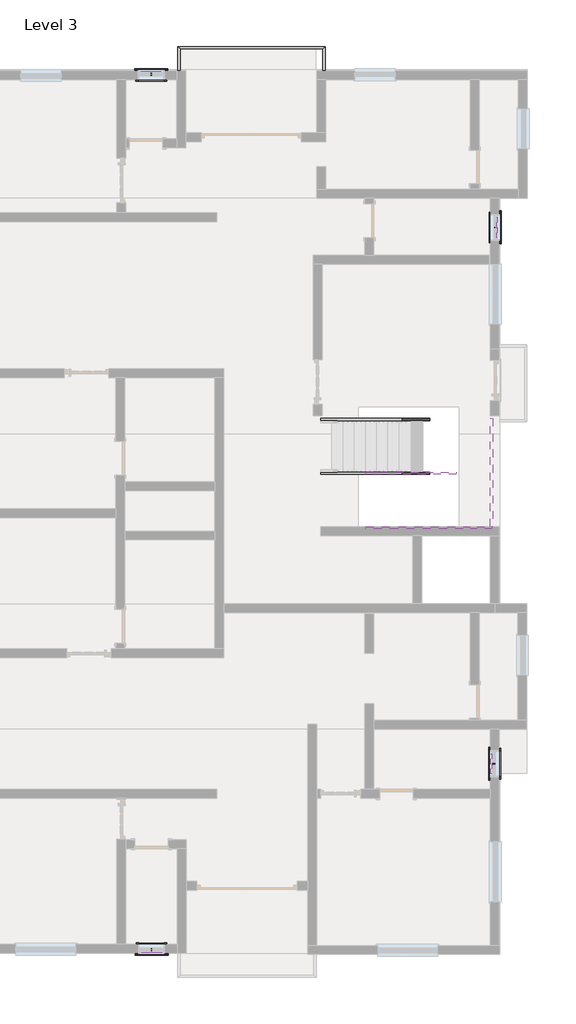
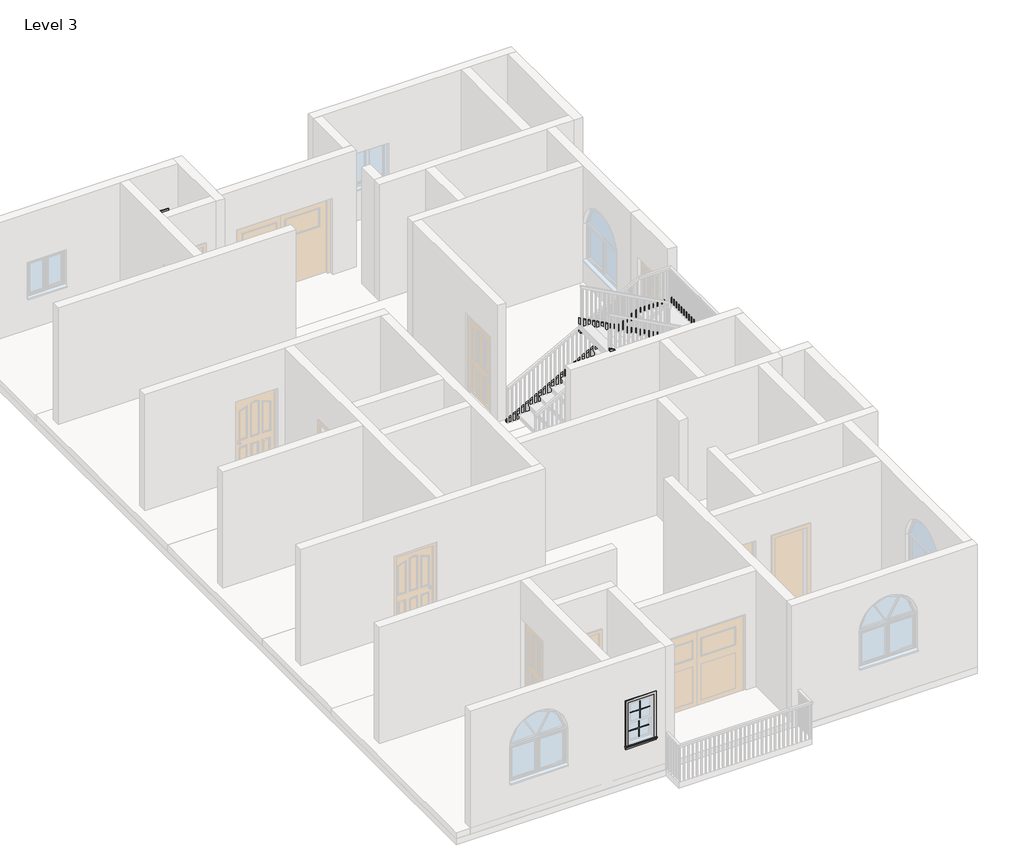
# One storey, part 7 of 7: 16 proxies, 5 members, 1 railing.
"""IFC4 building model written with IfcOpenShell, lengths in millimetres."""

from ifc_helpers import new_model, si_unit, frame, origin, place, context, project, spatial, polyline, outline, extrude, faceted_brep, transform, mapped, element, save
from components import muntin_pattern_2x2_muntin_pattern_2x2_eba6c5fb, trim_window_exterior_flat_with_sill_278e6a94, trim_window_interior_flat_picture_frame_e9fd5f45

model = new_model("IFC4")

# Units and contexts
model_context = context("Model", 3, world=origin())
ifc_project = project(units=[si_unit("LENGTHUNIT", "METRE", prefix="MILLI")], contexts=[model_context])

# Site, building, storey
site = spatial("IfcSite", under=ifc_project)
building = spatial("IfcBuilding", under=site)
storey = spatial("IfcBuildingStorey", under=building, Name="Level 3", Elevation=6096.0)

# Proxies
placement = place(None, origin())
muntin_pattern_2x2_muntin_pattern_2x2_shape = muntin_pattern_2x2_muntin_pattern_2x2_eba6c5fb(model_context)
element("IfcBuildingElementProxy", 1, Name="Muntin Pattern_2x2 : Muntin Pattern_2x2", ObjectType="Muntin Pattern_2x2 : Muntin Pattern_2x2", at=placement, inside=storey, context=model_context, shape_type="MappedRepresentation", body=[
    mapped(muntin_pattern_2x2_muntin_pattern_2x2_shape, transform((5828.2640963, 5846.2962251, 7566.025), x_axis=(0.0, -1.0, 0.0), y_axis=(1.0, 0.0, 0.0), z_axis=(0.0, 0.0, 1.0))),
])
element("IfcBuildingElementProxy", 2, Name="Muntin Pattern_2x2 : Muntin Pattern_2x2", ObjectType="Muntin Pattern_2x2 : Muntin Pattern_2x2", at=placement, inside=storey, context=model_context, shape_type="MappedRepresentation", body=[
    mapped(muntin_pattern_2x2_muntin_pattern_2x2_shape, transform((5783.8140963, 5846.2962251, 7086.6), x_axis=(0.0, -1.0, 0.0), y_axis=(1.0, 0.0, 0.0), z_axis=(0.0, 0.0, 1.0))),
])
element("IfcBuildingElementProxy", 3, Name="Muntin Pattern_2x2 : Muntin Pattern_2x2", ObjectType="Muntin Pattern_2x2 : Muntin Pattern_2x2", at=placement, inside=storey, context=model_context, shape_type="MappedRepresentation", body=[
    mapped(muntin_pattern_2x2_muntin_pattern_2x2_shape, transform((5694.9140963, -6313.9537749, 7566.025), x_axis=(0.0, 1.0, 0.0), y_axis=(-1.0, 0.0, 0.0), z_axis=(0.0, 0.0, 1.0))),
])
element("IfcBuildingElementProxy", 4, Name="Muntin Pattern_2x2 : Muntin Pattern_2x2", ObjectType="Muntin Pattern_2x2 : Muntin Pattern_2x2", at=placement, inside=storey, context=model_context, shape_type="MappedRepresentation", body=[
    mapped(muntin_pattern_2x2_muntin_pattern_2x2_shape, transform((5739.3640963, -6313.9537749, 7086.6), x_axis=(0.0, 1.0, 0.0), y_axis=(-1.0, 0.0, 0.0), z_axis=(0.0, 0.0, 1.0))),
])
element("IfcBuildingElementProxy", 5, Name="Muntin Pattern_2x2 : Muntin Pattern_2x2", ObjectType="Muntin Pattern_2x2 : Muntin Pattern_2x2", at=placement, inside=storey, context=model_context, shape_type="MappedRepresentation", body=[
    mapped(muntin_pattern_2x2_muntin_pattern_2x2_shape, transform((-2029.8609037, 9366.9277313, 7566.025), x_axis=(1.0, 0.0, 0.0), y_axis=(0.0, 1.0, 0.0), z_axis=(0.0, 0.0, 1.0))),
])
element("IfcBuildingElementProxy", 6, Name="Muntin Pattern_2x2 : Muntin Pattern_2x2", ObjectType="Muntin Pattern_2x2 : Muntin Pattern_2x2", at=placement, inside=storey, context=model_context, shape_type="MappedRepresentation", body=[
    mapped(muntin_pattern_2x2_muntin_pattern_2x2_shape, transform((-2029.8609037, 9322.4777313, 7086.6), x_axis=(1.0, 0.0, 0.0), y_axis=(0.0, 1.0, 0.0), z_axis=(0.0, 0.0, 1.0))),
])
element("IfcBuildingElementProxy", 7, Name="Muntin Pattern_2x2 : Muntin Pattern_2x2", ObjectType="Muntin Pattern_2x2 : Muntin Pattern_2x2", at=placement, inside=storey, context=model_context, shape_type="MappedRepresentation", body=[
    mapped(muntin_pattern_2x2_muntin_pattern_2x2_shape, transform((-2023.5109037, -10577.9787749, 7566.025), x_axis=(-1.0, 0.0, 0.0), y_axis=(0.0, -1.0, 0.0), z_axis=(0.0, 0.0, 1.0))),
])
element("IfcBuildingElementProxy", 8, Name="Muntin Pattern_2x2 : Muntin Pattern_2x2", ObjectType="Muntin Pattern_2x2 : Muntin Pattern_2x2", at=placement, inside=storey, context=model_context, shape_type="MappedRepresentation", body=[
    mapped(muntin_pattern_2x2_muntin_pattern_2x2_shape, transform((-2023.5109037, -10533.5287749, 7086.6), x_axis=(-1.0, 0.0, 0.0), y_axis=(0.0, -1.0, 0.0), z_axis=(0.0, 0.0, 1.0))),
])
trim_window_exterior_flat_with_sill_shape = trim_window_exterior_flat_with_sill_278e6a94(model_context)
element("IfcBuildingElementProxy", 9, Name="Trim-Window-Exterior-Flat : with Sill", ObjectType="Trim-Window-Exterior-Flat : with Sill", at=placement, inside=storey, context=model_context, shape_type="MappedRepresentation", body=[
    mapped(trim_window_exterior_flat_with_sill_shape, transform((5863.1890963, 5846.2962251, 8077.2), x_axis=(0.0, 1.0, 0.0), y_axis=(0.0, 0.0, 1.0), z_axis=(1.0, 0.0, 0.0))),
])
element("IfcBuildingElementProxy", 10, Name="Trim-Window-Exterior-Flat : with Sill", ObjectType="Trim-Window-Exterior-Flat : with Sill", at=placement, inside=storey, context=model_context, shape_type="MappedRepresentation", body=[
    mapped(trim_window_exterior_flat_with_sill_shape, transform((5659.9890963, -6313.9537749, 8077.2), x_axis=(0.0, -1.0, 0.0), y_axis=(0.0, 0.0, 1.0), z_axis=(-1.0, 0.0, 0.0))),
])
element("IfcBuildingElementProxy", 11, Name="Trim-Window-Exterior-Flat : with Sill", ObjectType="Trim-Window-Exterior-Flat : with Sill", at=placement, inside=storey, context=model_context, shape_type="MappedRepresentation", body=[
    mapped(trim_window_exterior_flat_with_sill_shape, transform((-2029.8609037, 9401.8527313, 8077.2), x_axis=(-1.0, 0.0, 0.0), y_axis=(0.0, 0.0, 1.0), z_axis=(0.0, 1.0, 0.0))),
])
element("IfcBuildingElementProxy", 12, Name="Trim-Window-Exterior-Flat : with Sill", ObjectType="Trim-Window-Exterior-Flat : with Sill", at=placement, inside=storey, context=model_context, shape_type="MappedRepresentation", body=[
    mapped(trim_window_exterior_flat_with_sill_shape, transform((-2023.5109037, -10612.9037749, 8077.2), x_axis=(1.0, 0.0, 0.0), y_axis=(0.0, 0.0, 1.0), z_axis=(0.0, -1.0, 0.0))),
])
trim_window_interior_flat_picture_frame_shape = trim_window_interior_flat_picture_frame_e9fd5f45(model_context)
element("IfcBuildingElementProxy", 13, Name="Trim-Window-Interior-Flat : Picture Frame", ObjectType="Trim-Window-Interior-Flat : Picture Frame", at=placement, inside=storey, context=model_context, shape_type="MappedRepresentation", body=[
    mapped(trim_window_interior_flat_picture_frame_shape, transform((5659.9890963, 5846.2962251, 8077.2), x_axis=(0.0, -1.0, 0.0), y_axis=(0.0, 0.0, 1.0), z_axis=(-1.0, 0.0, 0.0))),
])
element("IfcBuildingElementProxy", 14, Name="Trim-Window-Interior-Flat : Picture Frame", ObjectType="Trim-Window-Interior-Flat : Picture Frame", at=placement, inside=storey, context=model_context, shape_type="MappedRepresentation", body=[
    mapped(trim_window_interior_flat_picture_frame_shape, transform((5863.1890963, -6313.9537749, 8077.2), x_axis=(0.0, 1.0, 0.0), y_axis=(0.0, 0.0, 1.0), z_axis=(1.0, 0.0, 0.0))),
])
element("IfcBuildingElementProxy", 15, Name="Trim-Window-Interior-Flat : Picture Frame", ObjectType="Trim-Window-Interior-Flat : Picture Frame", at=placement, inside=storey, context=model_context, shape_type="MappedRepresentation", body=[
    mapped(trim_window_interior_flat_picture_frame_shape, transform((-2029.8609037, 9198.6527313, 8077.2), x_axis=(1.0, 0.0, 0.0), y_axis=(0.0, 0.0, 1.0), z_axis=(0.0, -1.0, 0.0))),
])
element("IfcBuildingElementProxy", 16, Name="Trim-Window-Interior-Flat : Picture Frame", ObjectType="Trim-Window-Interior-Flat : Picture Frame", at=placement, inside=storey, context=model_context, shape_type="MappedRepresentation", body=[
    mapped(trim_window_interior_flat_picture_frame_shape, transform((-2023.5109037, -10409.7037749, 8077.2), x_axis=(-1.0, 0.0, 0.0), y_axis=(0.0, 0.0, 1.0), z_axis=(0.0, 1.0, 0.0))),
])

# Members
element("IfcMember", 17, ObjectType="Stringer - 2\" Width", at=placement, inside=storey, context=model_context, shape_type="SweptSolid", body=[
    extrude(outline(polyline([(6303.4423129, 1811.8890963), (6096.0, 1811.8890963), (6096.0, 2068.9379367), (7973.2909091, 5536.6829612), (7973.2909091, 4896.4452154), (6303.4423129, 1811.8890963)])), frame((0.0, 1464.7962251, 0.0), z_axis=(0.0, 1.0, 0.0), x_axis=(0.0, 0.0, 1.0)), (0.0, 0.0, 1.0), 50.8),
])
element("IfcMember", 18, ObjectType="Stringer - 2\" Width", at=placement, inside=storey, context=model_context, shape_type="SweptSolid", body=[
    extrude(outline(polyline([(5659.9890963, 1515.5962251), (5710.7890963, 1515.5962251), (5710.7890963, -935.5037749), (5659.9890963, -935.5037749), (5659.9890963, 1515.5962251)])), frame((0.0, 0.0, 7668.4909091), z_axis=(0.0, 0.0, 1.0), x_axis=(1.0, 0.0, 0.0)), (0.0, 0.0, 1.0), 304.8),
])
element("IfcMember", 19, ObjectType="Stringer - 2\" Width", at=placement, inside=storey, context=model_context, shape_type="SweptSolid", body=[
    extrude(outline(polyline([(7668.4909091, 5687.6636359), (9210.0362324, 2827.8890963), (8863.7736638, 2827.8890963), (7668.4909091, 5045.2998579), (7668.4909091, 5687.6636359)])), frame((0.0, -986.3037749, 0.0), z_axis=(0.0, 1.0, 0.0), x_axis=(0.0, 0.0, 1.0)), (0.0, 0.0, 1.0), 50.8),
])
element("IfcMember", 20, ObjectType="Stringer - 2\" Width", at=placement, inside=storey, context=model_context, shape_type="SweptSolid", body=[
    extrude(outline(polyline([(6303.4423129, 1811.8890963), (6096.0, 1811.8890963), (6096.0, 2068.9379367), (7590.8485088, 4830.2326586), (7937.4462232, 4830.2326586), (6303.4423129, 1811.8890963)])), frame((0.0, 245.5962251, 0.0), z_axis=(0.0, 1.0, 0.0), x_axis=(0.0, 0.0, 1.0)), (0.0, 0.0, 1.0), 50.8),
])
element("IfcMember", 21, ObjectType="Stringer - 2\" Width", at=placement, inside=storey, context=model_context, shape_type="SweptSolid", body=[
    extrude(outline(polyline([(7757.0382157, 4881.0326586), (8103.3007843, 4881.0326586), (9210.0362324, 2827.8890963), (8863.7736638, 2827.8890963), (7757.0382157, 4881.0326586)])), frame((0.0, 245.5962251, 0.0), z_axis=(0.0, 1.0, 0.0), x_axis=(0.0, 0.0, 1.0)), (0.0, 0.0, 1.0), 50.8),
])

# Railing
element("IfcRailing", 22, ObjectType="Handrail - Rectangular", at=placement, inside=storey, context=model_context, shape_type="SolidModel", body=[
    faceted_brep([(-1426.6109037, 9402.2962251, 7010.4), (-1426.6109037, 9402.2962251, 6959.6), (-1375.8109037, 9402.2962251, 6959.6), (-1375.8109037, 9402.2962251, 7010.4), (-1426.6109037, 9948.3962251, 7010.4), (-1426.6109037, 9948.3962251, 6959.6), (-1375.8109037, 9897.5962251, 6959.6), (-1375.8109037, 9897.5962251, 7010.4), (1913.4890963, 9948.3962251, 7010.4), (1913.4890963, 9948.3962251, 6959.6), (1862.6890963, 9897.5962251, 6959.6), (1862.6890963, 9897.5962251, 7010.4), (1913.4890963, 9402.2962251, 7010.4), (1862.6890963, 9402.2962251, 7010.4), (1862.6890963, 9402.2962251, 6959.6), (1913.4890963, 9402.2962251, 6959.6)], [[[0, 1, 2, 3]], [[1, 0, 4, 5]], [[2, 1, 5, 6]], [[3, 2, 6, 7]], [[0, 3, 7, 4]], [[5, 4, 8, 9]], [[6, 5, 9, 10]], [[7, 6, 10, 11]], [[4, 7, 11, 8]], [[12, 13, 14, 15]], [[9, 8, 12, 15]], [[10, 9, 15, 14]], [[11, 10, 14, 13]], [[8, 11, 13, 12]]]),
    extrude(outline(polyline([(1878.5640963, 9424.5212251), (1897.6140963, 9424.5212251), (1897.6140963, 9405.4712251), (1878.5640963, 9405.4712251), (1878.5640963, 9424.5212251)])), frame((0.0, 0.0, 6096.0), z_axis=(0.0, 0.0, 1.0), x_axis=(1.0, 0.0, 0.0)), (0.0, 0.0, 1.0), 863.6),
    extrude(outline(polyline([(1878.5640963, 9526.1212251), (1897.6140963, 9526.1212251), (1897.6140963, 9507.0712251), (1878.5640963, 9507.0712251), (1878.5640963, 9526.1212251)])), frame((0.0, 0.0, 6096.0), z_axis=(0.0, 0.0, 1.0), x_axis=(1.0, 0.0, 0.0)), (0.0, 0.0, 1.0), 863.6),
    extrude(outline(polyline([(1878.5640963, 9627.7212251), (1897.6140963, 9627.7212251), (1897.6140963, 9608.6712251), (1878.5640963, 9608.6712251), (1878.5640963, 9627.7212251)])), frame((0.0, 0.0, 6096.0), z_axis=(0.0, 0.0, 1.0), x_axis=(1.0, 0.0, 0.0)), (0.0, 0.0, 1.0), 863.6),
    extrude(outline(polyline([(1878.5640963, 9729.3212251), (1897.6140963, 9729.3212251), (1897.6140963, 9710.2712251), (1878.5640963, 9710.2712251), (1878.5640963, 9729.3212251)])), frame((0.0, 0.0, 6096.0), z_axis=(0.0, 0.0, 1.0), x_axis=(1.0, 0.0, 0.0)), (0.0, 0.0, 1.0), 863.6),
    extrude(outline(polyline([(1878.5640963, 9830.9212251), (1897.6140963, 9830.9212251), (1897.6140963, 9811.8712251), (1878.5640963, 9811.8712251), (1878.5640963, 9830.9212251)])), frame((0.0, 0.0, 6096.0), z_axis=(0.0, 0.0, 1.0), x_axis=(1.0, 0.0, 0.0)), (0.0, 0.0, 1.0), 863.6),
    extrude(outline(polyline([(1840.4640963, 9913.4712251), (1840.4640963, 9932.5212251), (1859.5140963, 9932.5212251), (1859.5140963, 9913.4712251), (1840.4640963, 9913.4712251)])), frame((0.0, 0.0, 6096.0), z_axis=(0.0, 0.0, 1.0), x_axis=(1.0, 0.0, 0.0)), (0.0, 0.0, 1.0), 863.6),
    extrude(outline(polyline([(1738.8640963, 9913.4712251), (1738.8640963, 9932.5212251), (1757.9140963, 9932.5212251), (1757.9140963, 9913.4712251), (1738.8640963, 9913.4712251)])), frame((0.0, 0.0, 6096.0), z_axis=(0.0, 0.0, 1.0), x_axis=(1.0, 0.0, 0.0)), (0.0, 0.0, 1.0), 863.6),
    extrude(outline(polyline([(1637.2640963, 9913.4712251), (1637.2640963, 9932.5212251), (1656.3140963, 9932.5212251), (1656.3140963, 9913.4712251), (1637.2640963, 9913.4712251)])), frame((0.0, 0.0, 6096.0), z_axis=(0.0, 0.0, 1.0), x_axis=(1.0, 0.0, 0.0)), (0.0, 0.0, 1.0), 863.6),
    extrude(outline(polyline([(1535.6640963, 9913.4712251), (1535.6640963, 9932.5212251), (1554.7140963, 9932.5212251), (1554.7140963, 9913.4712251), (1535.6640963, 9913.4712251)])), frame((0.0, 0.0, 6096.0), z_axis=(0.0, 0.0, 1.0), x_axis=(1.0, 0.0, 0.0)), (0.0, 0.0, 1.0), 863.6),
    extrude(outline(polyline([(1434.0640963, 9913.4712251), (1434.0640963, 9932.5212251), (1453.1140963, 9932.5212251), (1453.1140963, 9913.4712251), (1434.0640963, 9913.4712251)])), frame((0.0, 0.0, 6096.0), z_axis=(0.0, 0.0, 1.0), x_axis=(1.0, 0.0, 0.0)), (0.0, 0.0, 1.0), 863.6),
    extrude(outline(polyline([(1332.4640963, 9913.4712251), (1332.4640963, 9932.5212251), (1351.5140963, 9932.5212251), (1351.5140963, 9913.4712251), (1332.4640963, 9913.4712251)])), frame((0.0, 0.0, 6096.0), z_axis=(0.0, 0.0, 1.0), x_axis=(1.0, 0.0, 0.0)), (0.0, 0.0, 1.0), 863.6),
    extrude(outline(polyline([(1230.8640963, 9913.4712251), (1230.8640963, 9932.5212251), (1249.9140963, 9932.5212251), (1249.9140963, 9913.4712251), (1230.8640963, 9913.4712251)])), frame((0.0, 0.0, 6096.0), z_axis=(0.0, 0.0, 1.0), x_axis=(1.0, 0.0, 0.0)), (0.0, 0.0, 1.0), 863.6),
    extrude(outline(polyline([(1129.2640963, 9913.4712251), (1129.2640963, 9932.5212251), (1148.3140963, 9932.5212251), (1148.3140963, 9913.4712251), (1129.2640963, 9913.4712251)])), frame((0.0, 0.0, 6096.0), z_axis=(0.0, 0.0, 1.0), x_axis=(1.0, 0.0, 0.0)), (0.0, 0.0, 1.0), 863.6),
    extrude(outline(polyline([(1027.6640963, 9913.4712251), (1027.6640963, 9932.5212251), (1046.7140963, 9932.5212251), (1046.7140963, 9913.4712251), (1027.6640963, 9913.4712251)])), frame((0.0, 0.0, 6096.0), z_axis=(0.0, 0.0, 1.0), x_axis=(1.0, 0.0, 0.0)), (0.0, 0.0, 1.0), 863.6),
    extrude(outline(polyline([(926.0640963, 9913.4712251), (926.0640963, 9932.5212251), (945.1140963, 9932.5212251), (945.1140963, 9913.4712251), (926.0640963, 9913.4712251)])), frame((0.0, 0.0, 6096.0), z_axis=(0.0, 0.0, 1.0), x_axis=(1.0, 0.0, 0.0)), (0.0, 0.0, 1.0), 863.6),
    extrude(outline(polyline([(824.4640963, 9913.4712251), (824.4640963, 9932.5212251), (843.5140963, 9932.5212251), (843.5140963, 9913.4712251), (824.4640963, 9913.4712251)])), frame((0.0, 0.0, 6096.0), z_axis=(0.0, 0.0, 1.0), x_axis=(1.0, 0.0, 0.0)), (0.0, 0.0, 1.0), 863.6),
    extrude(outline(polyline([(722.8640963, 9913.4712251), (722.8640963, 9932.5212251), (741.9140963, 9932.5212251), (741.9140963, 9913.4712251), (722.8640963, 9913.4712251)])), frame((0.0, 0.0, 6096.0), z_axis=(0.0, 0.0, 1.0), x_axis=(1.0, 0.0, 0.0)), (0.0, 0.0, 1.0), 863.6),
    extrude(outline(polyline([(621.2640963, 9913.4712251), (621.2640963, 9932.5212251), (640.3140963, 9932.5212251), (640.3140963, 9913.4712251), (621.2640963, 9913.4712251)])), frame((0.0, 0.0, 6096.0), z_axis=(0.0, 0.0, 1.0), x_axis=(1.0, 0.0, 0.0)), (0.0, 0.0, 1.0), 863.6),
    extrude(outline(polyline([(519.6640963, 9913.4712251), (519.6640963, 9932.5212251), (538.7140963, 9932.5212251), (538.7140963, 9913.4712251), (519.6640963, 9913.4712251)])), frame((0.0, 0.0, 6096.0), z_axis=(0.0, 0.0, 1.0), x_axis=(1.0, 0.0, 0.0)), (0.0, 0.0, 1.0), 863.6),
    extrude(outline(polyline([(418.0640963, 9913.4712251), (418.0640963, 9932.5212251), (437.1140963, 9932.5212251), (437.1140963, 9913.4712251), (418.0640963, 9913.4712251)])), frame((0.0, 0.0, 6096.0), z_axis=(0.0, 0.0, 1.0), x_axis=(1.0, 0.0, 0.0)), (0.0, 0.0, 1.0), 863.6),
    extrude(outline(polyline([(316.4640963, 9913.4712251), (316.4640963, 9932.5212251), (335.5140963, 9932.5212251), (335.5140963, 9913.4712251), (316.4640963, 9913.4712251)])), frame((0.0, 0.0, 6096.0), z_axis=(0.0, 0.0, 1.0), x_axis=(1.0, 0.0, 0.0)), (0.0, 0.0, 1.0), 863.6),
    extrude(outline(polyline([(214.8640963, 9913.4712251), (214.8640963, 9932.5212251), (233.9140963, 9932.5212251), (233.9140963, 9913.4712251), (214.8640963, 9913.4712251)])), frame((0.0, 0.0, 6096.0), z_axis=(0.0, 0.0, 1.0), x_axis=(1.0, 0.0, 0.0)), (0.0, 0.0, 1.0), 863.6),
    extrude(outline(polyline([(113.2640963, 9913.4712251), (113.2640963, 9932.5212251), (132.3140963, 9932.5212251), (132.3140963, 9913.4712251), (113.2640963, 9913.4712251)])), frame((0.0, 0.0, 6096.0), z_axis=(0.0, 0.0, 1.0), x_axis=(1.0, 0.0, 0.0)), (0.0, 0.0, 1.0), 863.6),
    extrude(outline(polyline([(11.6640963, 9913.4712251), (11.6640963, 9932.5212251), (30.7140963, 9932.5212251), (30.7140963, 9913.4712251), (11.6640963, 9913.4712251)])), frame((0.0, 0.0, 6096.0), z_axis=(0.0, 0.0, 1.0), x_axis=(1.0, 0.0, 0.0)), (0.0, 0.0, 1.0), 863.6),
    extrude(outline(polyline([(-89.9359037, 9913.4712251), (-89.9359037, 9932.5212251), (-70.8859037, 9932.5212251), (-70.8859037, 9913.4712251), (-89.9359037, 9913.4712251)])), frame((0.0, 0.0, 6096.0), z_axis=(0.0, 0.0, 1.0), x_axis=(1.0, 0.0, 0.0)), (0.0, 0.0, 1.0), 863.6),
    extrude(outline(polyline([(-191.5359037, 9913.4712251), (-191.5359037, 9932.5212251), (-172.4859037, 9932.5212251), (-172.4859037, 9913.4712251), (-191.5359037, 9913.4712251)])), frame((0.0, 0.0, 6096.0), z_axis=(0.0, 0.0, 1.0), x_axis=(1.0, 0.0, 0.0)), (0.0, 0.0, 1.0), 863.6),
    extrude(outline(polyline([(-293.1359037, 9913.4712251), (-293.1359037, 9932.5212251), (-274.0859037, 9932.5212251), (-274.0859037, 9913.4712251), (-293.1359037, 9913.4712251)])), frame((0.0, 0.0, 6096.0), z_axis=(0.0, 0.0, 1.0), x_axis=(1.0, 0.0, 0.0)), (0.0, 0.0, 1.0), 863.6),
    extrude(outline(polyline([(-394.7359037, 9913.4712251), (-394.7359037, 9932.5212251), (-375.6859037, 9932.5212251), (-375.6859037, 9913.4712251), (-394.7359037, 9913.4712251)])), frame((0.0, 0.0, 6096.0), z_axis=(0.0, 0.0, 1.0), x_axis=(1.0, 0.0, 0.0)), (0.0, 0.0, 1.0), 863.6),
    extrude(outline(polyline([(-496.3359037, 9913.4712251), (-496.3359037, 9932.5212251), (-477.2859037, 9932.5212251), (-477.2859037, 9913.4712251), (-496.3359037, 9913.4712251)])), frame((0.0, 0.0, 6096.0), z_axis=(0.0, 0.0, 1.0), x_axis=(1.0, 0.0, 0.0)), (0.0, 0.0, 1.0), 863.6),
    extrude(outline(polyline([(-597.9359037, 9913.4712251), (-597.9359037, 9932.5212251), (-578.8859037, 9932.5212251), (-578.8859037, 9913.4712251), (-597.9359037, 9913.4712251)])), frame((0.0, 0.0, 6096.0), z_axis=(0.0, 0.0, 1.0), x_axis=(1.0, 0.0, 0.0)), (0.0, 0.0, 1.0), 863.6),
    extrude(outline(polyline([(-699.5359037, 9913.4712251), (-699.5359037, 9932.5212251), (-680.4859037, 9932.5212251), (-680.4859037, 9913.4712251), (-699.5359037, 9913.4712251)])), frame((0.0, 0.0, 6096.0), z_axis=(0.0, 0.0, 1.0), x_axis=(1.0, 0.0, 0.0)), (0.0, 0.0, 1.0), 863.6),
    extrude(outline(polyline([(-801.1359037, 9913.4712251), (-801.1359037, 9932.5212251), (-782.0859037, 9932.5212251), (-782.0859037, 9913.4712251), (-801.1359037, 9913.4712251)])), frame((0.0, 0.0, 6096.0), z_axis=(0.0, 0.0, 1.0), x_axis=(1.0, 0.0, 0.0)), (0.0, 0.0, 1.0), 863.6),
    extrude(outline(polyline([(-902.7359037, 9913.4712251), (-902.7359037, 9932.5212251), (-883.6859037, 9932.5212251), (-883.6859037, 9913.4712251), (-902.7359037, 9913.4712251)])), frame((0.0, 0.0, 6096.0), z_axis=(0.0, 0.0, 1.0), x_axis=(1.0, 0.0, 0.0)), (0.0, 0.0, 1.0), 863.6),
    extrude(outline(polyline([(-1004.3359037, 9913.4712251), (-1004.3359037, 9932.5212251), (-985.2859037, 9932.5212251), (-985.2859037, 9913.4712251), (-1004.3359037, 9913.4712251)])), frame((0.0, 0.0, 6096.0), z_axis=(0.0, 0.0, 1.0), x_axis=(1.0, 0.0, 0.0)), (0.0, 0.0, 1.0), 863.6),
    extrude(outline(polyline([(-1105.9359037, 9913.4712251), (-1105.9359037, 9932.5212251), (-1086.8859037, 9932.5212251), (-1086.8859037, 9913.4712251), (-1105.9359037, 9913.4712251)])), frame((0.0, 0.0, 6096.0), z_axis=(0.0, 0.0, 1.0), x_axis=(1.0, 0.0, 0.0)), (0.0, 0.0, 1.0), 863.6),
    extrude(outline(polyline([(-1207.5359037, 9913.4712251), (-1207.5359037, 9932.5212251), (-1188.4859037, 9932.5212251), (-1188.4859037, 9913.4712251), (-1207.5359037, 9913.4712251)])), frame((0.0, 0.0, 6096.0), z_axis=(0.0, 0.0, 1.0), x_axis=(1.0, 0.0, 0.0)), (0.0, 0.0, 1.0), 863.6),
    extrude(outline(polyline([(-1309.1359037, 9913.4712251), (-1309.1359037, 9932.5212251), (-1290.0859037, 9932.5212251), (-1290.0859037, 9913.4712251), (-1309.1359037, 9913.4712251)])), frame((0.0, 0.0, 6096.0), z_axis=(0.0, 0.0, 1.0), x_axis=(1.0, 0.0, 0.0)), (0.0, 0.0, 1.0), 863.6),
    extrude(outline(polyline([(-1391.6859037, 9900.7712251), (-1410.7359037, 9900.7712251), (-1410.7359037, 9919.8212251), (-1391.6859037, 9919.8212251), (-1391.6859037, 9900.7712251)])), frame((0.0, 0.0, 6096.0), z_axis=(0.0, 0.0, 1.0), x_axis=(1.0, 0.0, 0.0)), (0.0, 0.0, 1.0), 863.6),
    extrude(outline(polyline([(-1391.6859037, 9799.1712251), (-1410.7359037, 9799.1712251), (-1410.7359037, 9818.2212251), (-1391.6859037, 9818.2212251), (-1391.6859037, 9799.1712251)])), frame((0.0, 0.0, 6096.0), z_axis=(0.0, 0.0, 1.0), x_axis=(1.0, 0.0, 0.0)), (0.0, 0.0, 1.0), 863.6),
    extrude(outline(polyline([(-1391.6859037, 9697.5712251), (-1410.7359037, 9697.5712251), (-1410.7359037, 9716.6212251), (-1391.6859037, 9716.6212251), (-1391.6859037, 9697.5712251)])), frame((0.0, 0.0, 6096.0), z_axis=(0.0, 0.0, 1.0), x_axis=(1.0, 0.0, 0.0)), (0.0, 0.0, 1.0), 863.6),
    extrude(outline(polyline([(-1391.6859037, 9595.9712251), (-1410.7359037, 9595.9712251), (-1410.7359037, 9615.0212251), (-1391.6859037, 9615.0212251), (-1391.6859037, 9595.9712251)])), frame((0.0, 0.0, 6096.0), z_axis=(0.0, 0.0, 1.0), x_axis=(1.0, 0.0, 0.0)), (0.0, 0.0, 1.0), 863.6),
    extrude(outline(polyline([(-1391.6859037, 9494.3712251), (-1410.7359037, 9494.3712251), (-1410.7359037, 9513.4212251), (-1391.6859037, 9513.4212251), (-1391.6859037, 9494.3712251)])), frame((0.0, 0.0, 6096.0), z_axis=(0.0, 0.0, 1.0), x_axis=(1.0, 0.0, 0.0)), (0.0, 0.0, 1.0), 863.6),
    extrude(outline(polyline([(1878.5640963, 9913.4712251), (1878.5640963, 9932.5212251), (1897.6140963, 9932.5212251), (1897.6140963, 9913.4712251), (1878.5640963, 9913.4712251)])), frame((0.0, 0.0, 6096.0), z_axis=(0.0, 0.0, 1.0), x_axis=(1.0, 0.0, 0.0)), (0.0, 0.0, 1.0), 863.6),
    extrude(outline(polyline([(-1391.6859037, 9913.4712251), (-1410.7359037, 9913.4712251), (-1410.7359037, 9932.5212251), (-1391.6859037, 9932.5212251), (-1391.6859037, 9913.4712251)])), frame((0.0, 0.0, 6096.0), z_axis=(0.0, 0.0, 1.0), x_axis=(1.0, 0.0, 0.0)), (0.0, 0.0, 1.0), 863.6),
    extrude(outline(polyline([(1878.5640963, 9421.3462251), (1897.6140963, 9421.3462251), (1897.6140963, 9402.2962251), (1878.5640963, 9402.2962251), (1878.5640963, 9421.3462251)])), frame((0.0, 0.0, 6096.0), z_axis=(0.0, 0.0, 1.0), x_axis=(1.0, 0.0, 0.0)), (0.0, 0.0, 1.0), 863.6),
    extrude(outline(polyline([(-1391.6859037, 9402.2962251), (-1410.7359037, 9402.2962251), (-1410.7359037, 9421.3462251), (-1391.6859037, 9421.3462251), (-1391.6859037, 9402.2962251)])), frame((0.0, 0.0, 6096.0), z_axis=(0.0, 0.0, 1.0), x_axis=(1.0, 0.0, 0.0)), (0.0, 0.0, 1.0), 863.6),
])

save(model, "model.ifc")

# Revit data of these elements
# Type "Muntin Pattern_2x2 : Muntin Pattern_2x2"
#   Width [instance default] = 4' - 0"
#   Thickness = 0' - 0 1/2"
#   Height [instance default] = 4' - 0"
#   Distance = 0' - 0 3/4"
#   Interior Material [instance default] = none
#   Exterior Material [instance default] = none
#   Default Elevation = 0
# Type "Trim-Window-Exterior-Flat : with Sill"
#   Trim Width = 0' - 2 1/4"
#   Trim Thickness_Picture Frame = 0' - 1 1/4"
#   Trim Thickness_with Sill = 0' - 0 3/4"
#   Sill Thickness = 0' - 1 1/4"
#   Opening Width [instance default] = 2' - 0"
#   Opening Height [instance default] = 3' - 0"
#   Default Elevation = 4' - 0"
#   Sill = yes
#   Picture Frame = no
#   Trim Material [instance default] = none
# Type "Trim-Window-Interior-Flat : Picture Frame"
#   Trim Thickness_Picture Frame = 0' - 1 1/4"
#   Trim Width = 0' - 2 1/4"
#   Trim Thickness_with Sill = 0' - 0 3/4"
#   Sill Thickness = 0' - 1 1/4"
#   Opening Width [instance default] = 2' - 0"
#   Opening Height [instance default] = 3' - 0"
#   Default Elevation = 4' - 0"
#   Sill = no
#   Picture Frame = yes
#   Trim Material [instance default] = none
# Type "Handrail - Rectangular"
#   Assembly Code = "C2010400"
#   built-in parameter 1008612 = 0.0416667 (stored number, unit not read)
#   built-in parameter 1008611 = 0.0416667 (stored number, unit not read)
#   built-in parameter 1008609 = 0.333333 (stored number, unit not read)
#   built-in parameter 1008604 = 0.166667 (stored number, unit not read)
#   built-in parameter 1008603 = 0.166667 (stored number, unit not read)
#   Railing Height = 3' - 0"
#   built-in parameter 1008630 = 2
#   built-in parameter 1008610 = 2
#   built-in parameter 1008618 = Baluster - Square : 3/4"
# Elements 1, 2, 3, 4, 5, 6, 7, 8 (IfcBuildingElementProxy, "Muntin Pattern_2x2 : Muntin Pattern_2x2")
#   Width = 1' - 6"
#   Height = 1' - 5 1/8"
#   Interior Material = Wood - Stained
#   Exterior Material = Clad - White
#   Phase Created = New Construction
#   Materials on its faces: "Clad - White", "Wood - Stained"
# Elements 9, 10, 11, 12 (IfcBuildingElementProxy, "Trim-Window-Exterior-Flat : with Sill")
#   Opening Width = 2' - 0"
#   Opening Height = 3' - 6"
#   Trim Material = Clad - White
#   Phase Created = New Construction
#   Materials on its faces: "Clad - White"
# Elements 13, 14, 15, 16 (IfcBuildingElementProxy, "Trim-Window-Interior-Flat : Picture Frame")
#   Opening Width = 2' - 0"
#   Opening Height = 3' - 6"
#   Trim Material = Wood - Stained
#   Phase Created = New Construction
#   Materials on its faces: "Wood - Stained"
# Elements 17, 18, 19, 20, 21 (IfcMember, "Stringer - 2\" Width")
#   Phase Created = New Construction
# Element 22 (IfcRailing, "Handrail - Rectangular")
#   Phase Created = New Construction
# Materials
#   "Clad - White": class "Wood", colour RGB 242 242 238, transparency 0, Cost = 0
#   "Wood - Stained": class "Wood", colour RGB 224 178 126, transparency 0, Cost = 0
